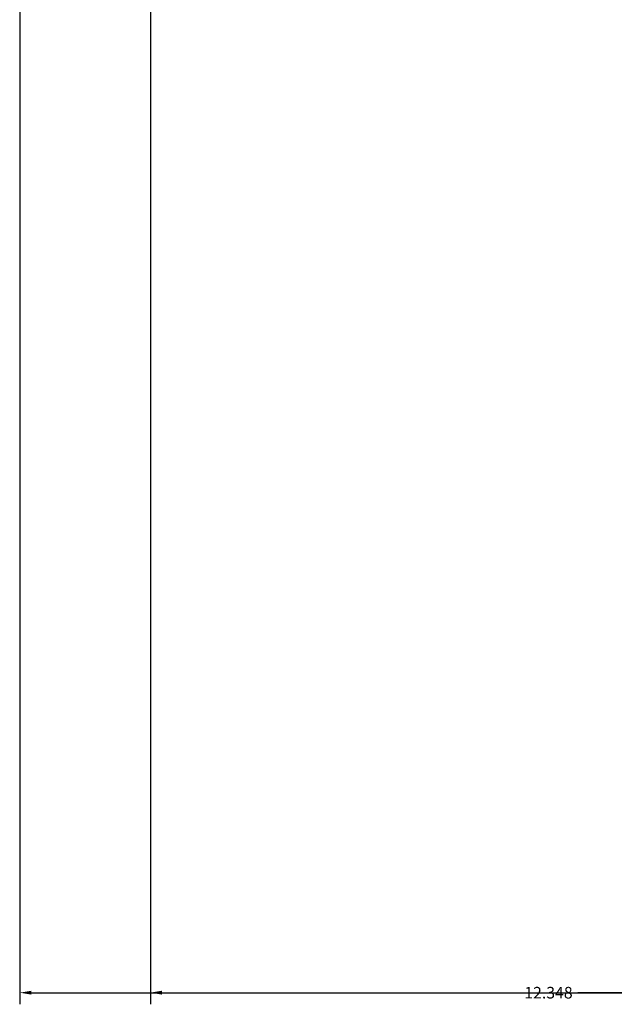
# Model space of a CAD drawing. Units: inches. Extents: x -6 to 289, y -8 to 323.
# Tile 1 of 107: x 9.94 to 19.16, y -8.39 to 6.88. Entities that reach past the tile are written whole.
import ezdxf

# ---------------------------------------------------------------- set-up
doc = ezdxf.new("R2010")
doc.units = ezdxf.units.IN
doc.header["$MEASUREMENT"] = 0
doc.layers.add('A-ANNO-DIMS', color=2, linetype='Continuous', lineweight=18)
doc.styles.get("Standard").update_dxf_attribs({"font": 'arial.ttf'})
doc.dimstyles.get("Standard").update_dxf_attribs({"dimtxt": 0.18, "dimasz": 0.18, "dimexe": 0.18, "dimexo": 0.0625, "dimgap": 0.09, "dimtad": 0, "dimtih": 1, "dimtoh": 1, "dimdec": 4, "dimzin": 0, "dimdsep": 46, "dimtxsty": 'Standard', "dimcen": 0.09, "dimadec": 0, "dimazin": 0, "dimtfac": 1, "dimtdec": 4, "dimtofl": 0, "dimtmove": 0, "dimatfit": 3, "dimfxl": 1, "dimtolj": 1, "dimtzin": 0, "dimarcsym": 0})

# ---------------------------------------------------------------- blocks, each defined once
blk = doc.blocks.new('*D16')
at = {"layer": 'A-ANNO-DIMS', "color": 0, "lineweight": -2, "transparency": 16777216}
for p, q in [((9.943, 68.37), (9.943, -8.391)), ((272.973, 68.37), (272.973, -8.391)), ((10.123, -8.211), (140.993, -8.211)), ((272.793, -8.211), (141.923, -8.211))]:
    blk.add_line(p, q, dxfattribs=at)
at = {"layer": 'A-ANNO-DIMS', "color": 0, "transparency": 16777216}
for points in [[(10.123, -8.181), (10.123, -8.241), (9.943, -8.211)], [(272.793, -8.181), (272.793, -8.241), (272.973, -8.211)]]:
    blk.add_solid(points, dxfattribs=at)
at = {"layer": 'Defpoints', "color": 0, "transparency": 16777216}
for p in [(9.943, 68.432), (272.973, 68.432), (272.973, -8.211)]:
    blk.add_point(p, dxfattribs=at)
at = {"layer": 'A-ANNO-DIMS', "color": 0, "transparency": 16777216, "insert": (141.458, -8.211), "char_height": 0.18, "attachment_point": 5}
blk.add_mtext('\\A1;263.03', dxfattribs=at)
blk = doc.blocks.new('*D50')
at = {"layer": 'A-ANNO-DIMS', "color": 0, "lineweight": -2, "transparency": 16777216}
for p, q in [((11.969, 7.226), (11.969, -8.391)), ((24.317, 7.226), (24.317, -8.391)), ((12.149, -8.211), (17.688, -8.211)), ((24.137, -8.211), (18.598, -8.211))]:
    blk.add_line(p, q, dxfattribs=at)
at = {"layer": 'A-ANNO-DIMS', "color": 0, "transparency": 16777216}
for points in [[(12.149, -8.181), (12.149, -8.241), (11.969, -8.211)], [(24.137, -8.181), (24.137, -8.241), (24.317, -8.211)]]:
    blk.add_solid(points, dxfattribs=at)
at = {"layer": 'Defpoints', "color": 0, "transparency": 16777216}
for p in [(11.969, 7.289), (24.317, 7.289), (24.317, -8.211)]:
    blk.add_point(p, dxfattribs=at)
at = {"layer": 'A-ANNO-DIMS', "color": 0, "transparency": 16777216, "insert": (18.143, -8.211), "char_height": 0.18, "attachment_point": 5}
blk.add_mtext('\\A1;12.348', dxfattribs=at)

msp = doc.modelspace()

# ---------------------------------------------------------------- dimensions: what is measured, and where the dimension line sits
at = {"layer": 'A-ANNO-DIMS'}
for base, p1, p2, override, picture, middle in [((272.9733, -8.2112), (9.943, 68.4322), (272.9733, 68.4322), {"dimdec": 2, "dimlfac": 1, "dimrnd": 0, "dimzin": 0, "dimdsep": 46, "dimlunit": 2}, '*D16', (141.4581, -8.2112)), ((24.317, -8.2112), (11.9692, 7.2888), (24.317, 7.2888), {"dimdec": 3, "dimlfac": 1, "dimrnd": 0, "dimzin": 0, "dimdsep": 46, "dimlunit": 2}, '*D50', (18.1431, -8.2112))]:
    dim = msp.add_linear_dim(base=base, p1=p1, p2=p2, dimstyle='Standard', override=override, dxfattribs=at)
    dim.commit()
    dim.dimension.update_dxf_attribs({"geometry": picture, "text_midpoint": middle})

doc.saveas('drawing.dxf')
